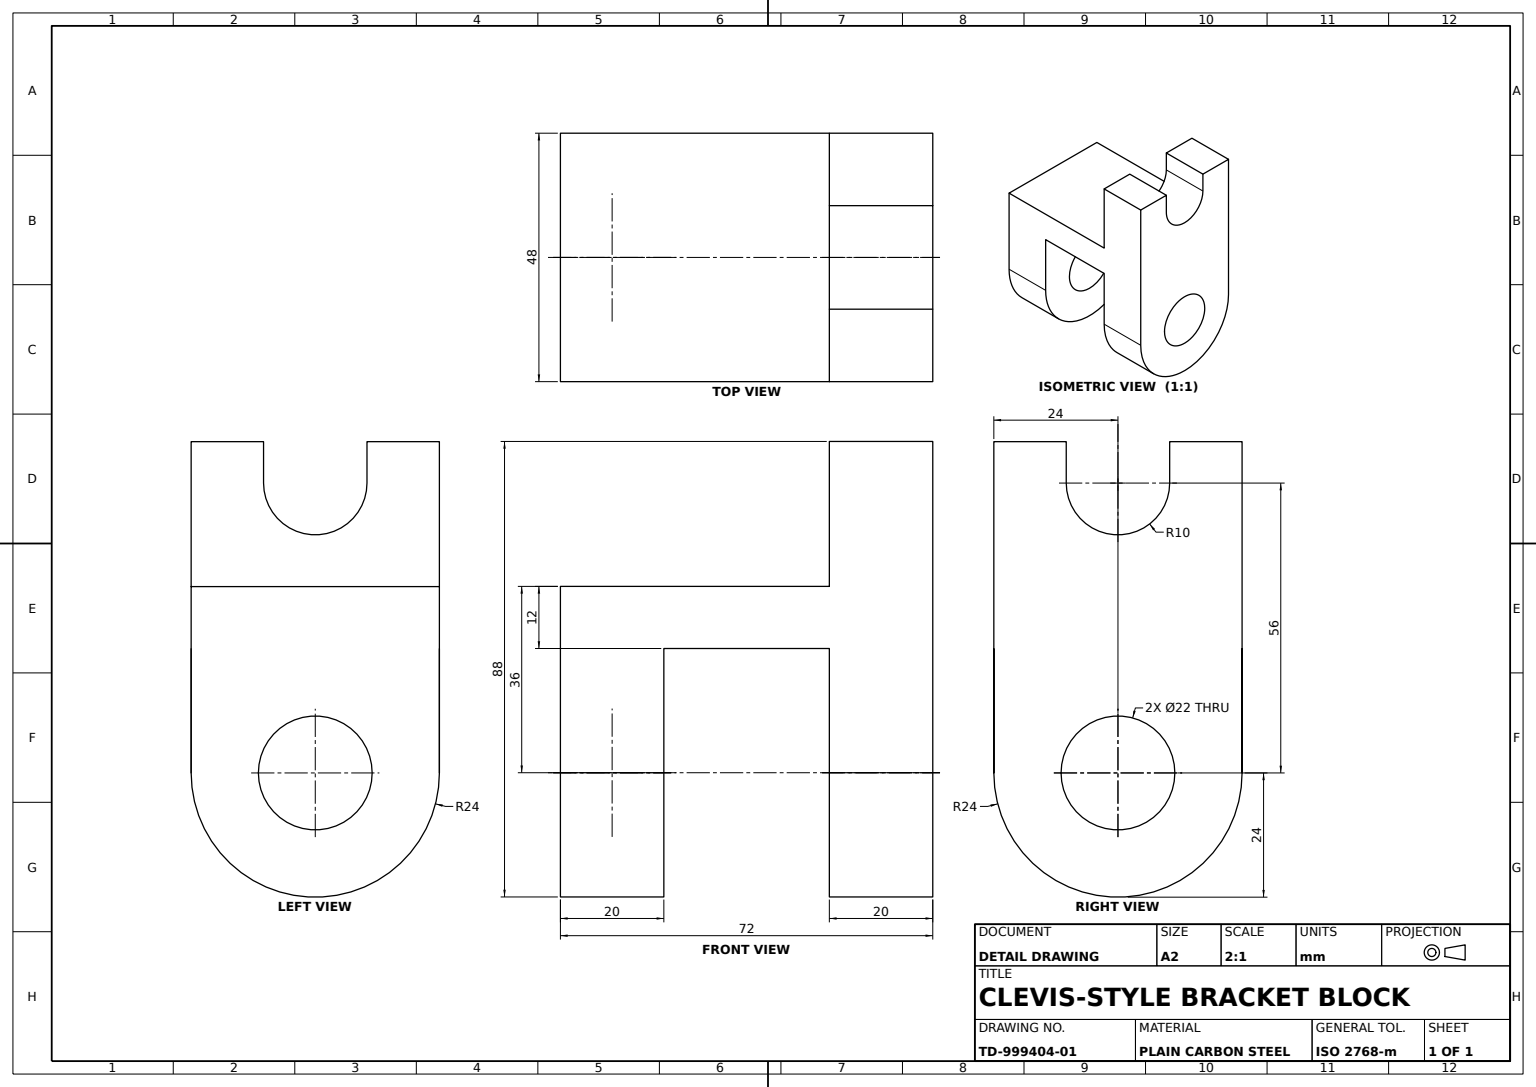
SolidWorks part; units mm, degrees
material "Plain Carbon Steel"
ref_plane "Front Plane" through (0, 0, 0) normal (0, 0, 1) x (1, 0, 0)
ref_plane "Top Plane" through (0, 0, 0) normal (0, 1, 0) x (1, 0, 0)
ref_plane "Right Plane" through (0, 0, 0) normal (1, 0, 0) x (0, 0, -1)
sketch "Front Lug Profile" plane through (0, 0, 0) normal (0, 0, 1) x (1, 0, 0)
  line L0 (24, 0) -> (24, 36)
  line L1 (-24, 0) -> (-24, 36)
  line L2 (-24, 36) -> (24, 36)
  arc A0 (-24, 0) -> (24, 0) centre (0, 0) ccw
  dimension "D1" = 24
  dimension "D2" = 36
extrude "Front Lug" add sketch "Front Lug Profile" against normal blind 20
ref_plane "Rear Lug Plane" through (0, 0, -52) normal (0, 0, -1) x (-1, 0, 0)
sketch "Rear Lug Profile" plane through (0, 0, -52) normal (0, 0, -1) x (-1, 0, 0)
  line L0 (-24, 0) -> (-24, 36)
  line L1 (-24, 36) -> (24, 36)
  line L2 (24, 36) -> (24, 0)
  arc A0 (-24, 0) -> (24, 0) centre (0, 0) ccw
extrude "Rear Lug" add sketch "Rear Lug Profile" along normal blind 20 separate body
sketch "Connecting Block Profile" plane through (0, 36, 0) normal (0, 1, 0) x (1, 0, 0)
  line L0 (-24, 20) -> (-24, 52)
  line L1 (-24, 52) -> (24, 52)
  line L2 (24, 52) -> (24, 20)
  line L3 (24, 20) -> (-24, 20)
extrude "Connecting Block" add sketch "Connecting Block Profile" against normal blind 12
sketch "Clevis Fork Profile" plane through (0, 0, -72) normal (0, 0, -1) x (-1, 0, 0)
  line L1 (10, 56) -> (10, 64)
  line L2 (10, 64) -> (24, 64)
  line L3 (24, 64) -> (24, 36)
  line L4 (24, 36) -> (-24, 36)
  line L5 (-10, 56) -> (-10, 64)
  line L6 (-10, 64) -> (-24, 64)
  line L7 (-24, 64) -> (-24, 36)
  arc A0 (-10, 56) -> (10, 56) centre (0, 56) ccw
  dimension "D1" = 20
  dimension "D2" = 20
  dimension "D3" = 56
  dimension "D4" = 28
  dimension "D5" = 28
extrude "Clevis Fork" add sketch "Clevis Fork Profile" against normal blind 20
sketch "Pin Hole Profile" plane through (0, 0, 0) normal (0, 0, 1) x (1, 0, 0)
  circle A0 centre (0, 0) radius 11
  dimension "D1" = 22
extrude "Pin Hole" cut sketch "Pin Hole Profile" against normal blind 99
